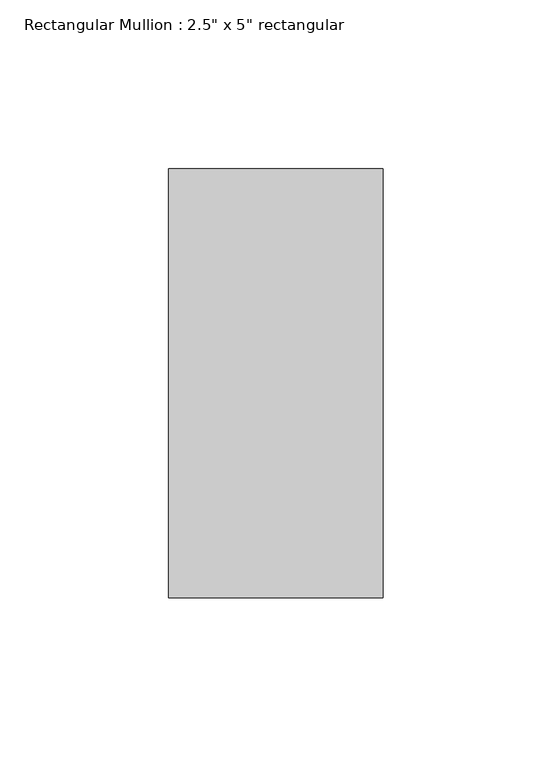
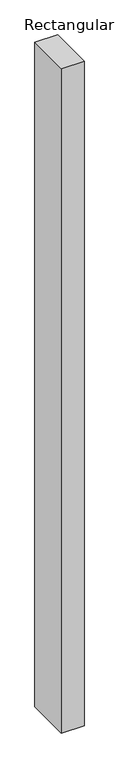
"""IFC4 building model written with IfcOpenShell, lengths in millimetres: member geometry."""

from ifc_helpers import new_model, si_unit, frame, origin, place, context, project, spatial, polyline, outline, extrude, source, transform, mapped, element, save


def member_5e69bd58(model_context):
    return source(origin(), model_context, "Body", "SweptSolid", [
        extrude(outline(polyline([(0.0, 63.5), (0.0, -63.5), (-63.5, -63.5), (-63.5, 63.5), (0.0, 63.5)])), frame((0.0, 0.0, -1954.7912729), z_axis=(0.0, 0.0, 1.0), x_axis=(1.0, 0.0, 0.0)), (0.0, 0.0, 1.0), 1954.7912729),
    ])


if __name__ == "__main__":
    model = new_model("IFC4")
    model_context = context("Model", 3, world=origin())
    ifc_project = project(units=[si_unit("LENGTHUNIT", "METRE", prefix="MILLI")], contexts=[model_context])
    site = spatial("IfcSite", under=ifc_project)
    building = spatial("IfcBuilding", under=site)
    placement = place(None, origin())
    member_shape = member_5e69bd58(model_context)
    element("IfcMember", 1, ObjectType="Rectangular Mullion : 2.5\" x 5\" rectangular", at=placement, inside=building, context=model_context, shape_type="MappedRepresentation", body=[
        mapped(member_shape, transform((0.0, 0.0, 0.0), x_axis=(1.0, 0.0, 0.0), y_axis=(0.0, 1.0, 0.0), z_axis=(0.0, 0.0, 1.0))),
    ])
    save(model, "model.ifc")

# Revit data of these elements
# Type "Rectangular Mullion : 2.5\" x 5\" rectangular"
#   built-in parameter 1007304 = 0.416667 (stored number, unit not read)
#   built-in parameter 1007301 = 0.104167 (stored number, unit not read)
#   built-in parameter 1007300 = 0.104167 (stored number, unit not read)
